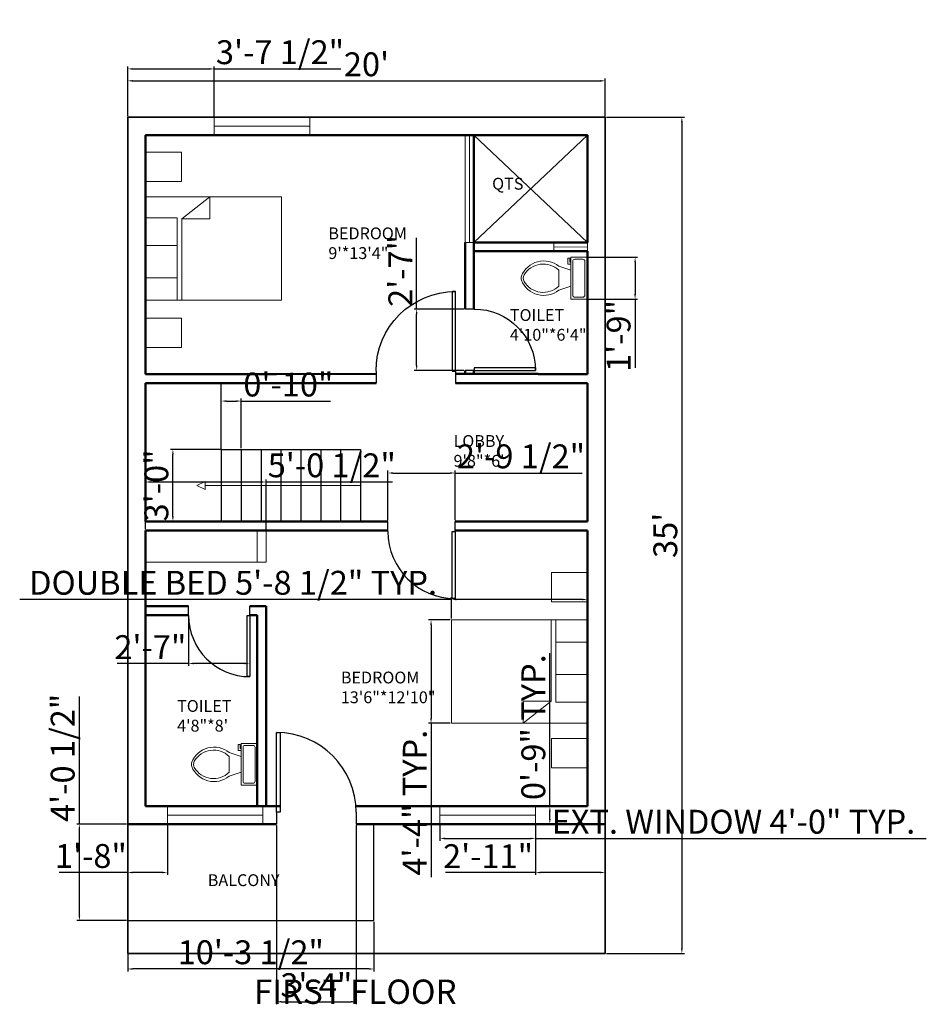
# Model space of a CAD drawing. Units: inches. Extents: x 2157 to 3060, y 2058 to 2553.
# Tile 2 of 2: x 2604 to 3060, y 2058 to 2553. Entities that reach past the tile are written whole.
import ezdxf

# ---------------------------------------------------------------- set-up
doc = ezdxf.new("R2010")
doc.units = ezdxf.units.IN
for name, color, linetype, lineweight in [('A-ANNO-DIMS', 2, 'Continuous', 18), ('A-ANNO-SYMB', 7, 'Continuous', 13), ('A-ANNO-TEXT', 7, 'Continuous', 35), ('A-AREA-IDEN', 7, 'Continuous', 18), ('A-FLOR', 7, 'Continuous', 25), ('A-FLOR-CASE', 32, 'Continuous', 20), ('A-FLOR-FIXT', 9, 'Continuous', 18), ('A-FLOR-STRS', 7, 'Continuous', 25), ('C-PROP', 7, 'Continuous', 35), ('DOOR', 2, 'Continuous', 25), ('FURNITURE', 32, 'Continuous', 18), ('WALL', 7, 'Continuous', 50), ('WINDOW', 130, 'Continuous', 18)]:
    doc.layers.add(name, color=color, linetype=linetype, lineweight=lineweight)
doc.styles.get("Standard").update_dxf_attribs({"font": 'arial.ttf'})
doc.dimstyles.new('ISO-25', dxfattribs={"dimtxt": 12, "dimasz": 2.5, "dimexe": 1.25, "dimexo": 0.625, "dimtad": 1, "dimdec": 0, "dimlunit": 4, "dimtxsty": 'Standard', "dimcen": 2.5, "dimadec": 0, "dimazin": 0, "dimtfac": 1, "dimtdec": 0, "dimtmove": 0, "dimatfit": 3, "dimfxl": 1, "dimarcsym": 0})

# ---------------------------------------------------------------- blocks, each defined once
blk = doc.blocks.new('*U2')
for p, q in [((0, 0), (0, -6)), ((40, 0), (40, -6))]:
    blk.add_line(p, q)
blk.add_lwpolyline([(0, 0), (0, 40), (1.75, 40), (1.75, 0)], close=True)
blk.add_arc((0, 0), 40, 0, 90)
blk = doc.blocks.new('*D7')
at = {"layer": 'A-ANNO-DIMS', "color": 0, "lineweight": -2, "transparency": 16777216}
for p, q in [((2658.57, 2504.59), (2658.57, 2523.53)), ((2898.57, 2504.59), (2898.57, 2523.53)), ((2661.07, 2522.28), (2896.07, 2522.28))]:
    blk.add_line(p, q, dxfattribs=at)
at = {"layer": 'A-ANNO-DIMS', "color": 0, "transparency": 16777216}
for points in [[(2661.07, 2522.7), (2661.07, 2521.86), (2658.57, 2522.28)], [(2896.07, 2522.7), (2896.07, 2521.86), (2898.57, 2522.28)]]:
    blk.add_solid(points, dxfattribs=at)
at = {"layer": 'Defpoints', "color": 0, "transparency": 16777216}
for p in [(2898.57, 2522.28), (2658.57, 2503.96), (2898.57, 2503.96)]:
    blk.add_point(p, dxfattribs=at)
at = {"layer": 'A-ANNO-DIMS', "color": 0, "transparency": 16777216, "insert": (2778.57, 2529.03), "char_height": 12, "attachment_point": 5}
blk.add_mtext("20'", dxfattribs=at)
blk = doc.blocks.new('*D8')
at = {"layer": 'A-ANNO-DIMS', "color": 0, "lineweight": -2, "transparency": 16777216}
for p, q in [((2899.2, 2503.96), (2938.3, 2503.96)), ((2937.05, 2501.46), (2937.05, 2086.46)), ((2899.2, 2083.96), (2938.3, 2083.96))]:
    blk.add_line(p, q, dxfattribs=at)
at = {"layer": 'A-ANNO-DIMS', "color": 0, "transparency": 16777216}
for points in [[(2936.63, 2501.46), (2937.47, 2501.46), (2937.05, 2503.96)], [(2936.63, 2086.46), (2937.47, 2086.46), (2937.05, 2083.96)]]:
    blk.add_solid(points, dxfattribs=at)
at = {"layer": 'Defpoints', "color": 0, "transparency": 16777216}
for p in [(2898.57, 2503.96), (2898.57, 2083.96), (2937.05, 2083.96)]:
    blk.add_point(p, dxfattribs=at)
at = {"layer": 'A-ANNO-DIMS', "color": 0, "transparency": 16777216, "insert": (2930.29, 2293.96), "char_height": 12, "attachment_point": 5, "rotation": 90}
blk.add_mtext("35'", dxfattribs=at)
blk = doc.blocks.new('*U4')
for p, q in [((9.5, -6), (9.5, -2)), ((-10, -8.5), (-8, -8.5)), ((-10, -9.5), (-10, -8.5)), ((-7, -9.5), (-10, -9.5)), ((-8, -8.5), (-8, -8)), ((-7, -8), (-7, -9.5)), ((-4, -8), (-6, -14)), ((4, -8), (6, -14)), ((4, -14), (-4, -14))]:
    blk.add_line(p, q)
blk.add_lwpolyline([(10.5, -8), (10.5, 0), (-10.5, 0), (-10.5, -8)], close=True)
for points in [[(-9.5, -2), (-9.5, -6)], [(8.5, -1), (-8.5, -1)], [(-8.5, -7), (8.5, -7)]]:
    blk.add_lwpolyline(points)
for centre, radius, start, end in [((-8.62, -1.88), 0.884, 81.8699, 188.1301), ((8.62, -1.88), 0.884, 351.8699, 98.1301), ((-8.62, -6.12), 0.884, 171.8699, 278.1301), ((8.62, -6.12), 0.884, 261.8699, 8.1301), ((3.52, -21.58), 12.17, 141.4691, 247.9714), ((4.2, -21.82), 11.33, 136.3677, 238.9468), ((-3.52, -21.58), 12.17, 292.0284, 38.5307), ((-4.2, -21.82), 11.33, 301.053, 43.6321), ((0, -27.88), 4, 245.7318, 294.2682), ((0, -29), 4, 254.8605, 285.1395)]:
    blk.add_arc(centre, radius, start, end)
blk = doc.blocks.new('BED-DOUBLE')
for p, q in [((18.2, 40.88), (32.33, 51.9)), ((32.33, 40.88), (32.33, 51.9)), ((18.2, 0), (18.2, 40.88)), ((18.2, 40.88), (32.33, 40.88)), ((0, 27.39), (15.88, 27.39)), ((0, 11.16), (15.88, 11.16))]:
    blk.add_line(p, q)
for points in [[(0, 0), (68.32, 0), (68.32, 51.9), (0, 51.9)], [(0, 0), (15.88, 0), (15.88, 41.3), (0, 41.3)]]:
    blk.add_lwpolyline(points, close=True)
blk = doc.blocks.new('NIGHTSTAND')
blk.add_lwpolyline([(0, 0), (17.99, 0), (17.99, 14.76), (0, 14.76)], close=True)
blk = doc.blocks.new('STAIR-FLIGHT')
for p, q in [((0, 36.14), (0, 69.5)), ((0, 36.14), (70, 36.14)), ((0, 36.14), (0, 0)), ((0, 36.14), (0, 0)), ((0, 36.14), (0, 0)), ((0, 36.14), (0, 0)), ((10, 36.14), (10, 0)), ((10, 36.14), (10, 0)), ((10, 36.14), (10, 0)), ((10, 36.14), (10, 0)), ((20, 36.14), (20, 0)), ((30, 36.14), (30, 0)), ((30, 36.14), (30, 0)), ((30, 36.14), (30, 0)), ((30, 36.14), (30, 0)), ((40, 36.14), (40, 0)), ((50, 36.14), (50, 0)), ((50, 36.14), (50, 0)), ((50, 36.14), (50, 0)), ((50, 36.14), (50, 0)), ((60, 36.14), (60, 0)), ((70, 36.14), (70, 0))]:
    blk.add_line(p, q)
blk = doc.blocks.new('STAIR-DIRECTION')
for p, q in [((4.17, 4), (0, 2)), ((0, 2), (4.17, 0)), ((4.17, 0), (4.17, 4)), ((82.21, 2), (4.17, 2)), ((4.17, 2), (4.17, 0))]:
    blk.add_line(p, q)
blk = doc.blocks.new('WIN-48IN-EXT')
for p, q in [((0, 4.5), (0, 9)), ((48, 4.5), (48, 9)), ((0, 4.5), (0, 0)), ((0, 4.5), (48, 4.5)), ((48, 4.5), (48, 0))]:
    blk.add_line(p, q)
blk = doc.blocks.new('OPEN-TO-SKY-MARK')
for p, q in [((57, 53.82), (0, 0)), ((57, 0), (0, 53.82))]:
    blk.add_line(p, q)
blk = doc.blocks.new('*D17')
at = {"layer": 'A-ANNO-DIMS', "color": 0, "lineweight": -2, "transparency": 16777216}
for p, q in [((2821.26, 2261.73), (2604.28, 2261.73)), ((2821.26, 2252.11), (2821.26, 2262.98)), ((2887.07, 2261.73), (2823.76, 2261.73)), ((2889.57, 2252.11), (2889.57, 2262.98))]:
    blk.add_line(p, q, dxfattribs=at)
at = {"layer": 'A-ANNO-DIMS', "color": 0, "transparency": 16777216}
for points in [[(2823.76, 2262.15), (2823.76, 2261.31), (2821.26, 2261.73)], [(2887.07, 2262.15), (2887.07, 2261.31), (2889.57, 2261.73)]]:
    blk.add_solid(points, dxfattribs=at)
at = {"layer": 'Defpoints', "color": 0, "transparency": 16777216}
for p in [(2821.26, 2261.73), (2821.26, 2251.48), (2889.57, 2251.48)]:
    blk.add_point(p, dxfattribs=at)
at = {"layer": 'A-ANNO-DIMS', "color": 0, "transparency": 16777216, "insert": (2711.52, 2268.57), "char_height": 12, "attachment_point": 5}
blk.add_mtext('DOUBLE BED 5\'-8 1/2" TYP.', dxfattribs=at)
blk = doc.blocks.new('*D18')
at = {"layer": 'A-ANNO-DIMS', "color": 0, "lineweight": -2, "transparency": 16777216}
for p, q in [((2820.63, 2251.48), (2809.76, 2251.48)), ((2811.01, 2248.98), (2811.01, 2202.09)), ((2820.63, 2199.59), (2809.76, 2199.59)), ((2811.01, 2199.59), (2811.01, 2122.21))]:
    blk.add_line(p, q, dxfattribs=at)
at = {"layer": 'A-ANNO-DIMS', "color": 0, "transparency": 16777216}
for points in [[(2810.59, 2248.98), (2811.43, 2248.98), (2811.01, 2251.48)], [(2810.59, 2202.09), (2811.43, 2202.09), (2811.01, 2199.59)]]:
    blk.add_solid(points, dxfattribs=at)
at = {"layer": 'Defpoints', "color": 0, "transparency": 16777216}
for p in [(2821.26, 2251.48), (2811.01, 2199.59), (2821.26, 2199.59)]:
    blk.add_point(p, dxfattribs=at)
at = {"layer": 'A-ANNO-DIMS', "color": 0, "transparency": 16777216, "insert": (2804.38, 2159.65), "char_height": 12, "attachment_point": 5, "rotation": 90}
blk.add_mtext('4\'-4" TYP.', dxfattribs=at)
blk = doc.blocks.new('*D19')
at = {"layer": 'A-ANNO-DIMS', "color": 0, "lineweight": -2, "transparency": 16777216}
for p, q in [((2815.5, 2148.26), (2815.5, 2140.43)), ((2863.5, 2148.26), (2863.5, 2140.43)), ((2818, 2141.68), (2861, 2141.68)), ((2863.5, 2141.68), (3059.9, 2141.68))]:
    blk.add_line(p, q, dxfattribs=at)
at = {"layer": 'A-ANNO-DIMS', "color": 0, "transparency": 16777216}
for points in [[(2818, 2142.1), (2818, 2141.26), (2815.5, 2141.68)], [(2861, 2142.1), (2861, 2141.26), (2863.5, 2141.68)]]:
    blk.add_solid(points, dxfattribs=at)
at = {"layer": 'Defpoints', "color": 0, "transparency": 16777216}
for p in [(2815.5, 2148.88), (2863.5, 2148.88), (2863.5, 2141.68)]:
    blk.add_point(p, dxfattribs=at)
at = {"layer": 'A-ANNO-DIMS', "color": 0, "transparency": 16777216, "insert": (2962.95, 2148.52), "char_height": 12, "attachment_point": 5}
blk.add_mtext('EXT. WINDOW 4\'-0" TYP.', dxfattribs=at)
blk = doc.blocks.new('*D20')
at = {"layer": 'A-ANNO-DIMS', "color": 0, "lineweight": -2, "transparency": 16777216}
for p, q in [((2870.7, 2157.88), (2870.7, 2234.78)), ((2864.13, 2157.88), (2871.95, 2157.88)), ((2870.7, 2151.38), (2870.7, 2155.38)), ((2864.13, 2148.88), (2871.95, 2148.88))]:
    blk.add_line(p, q, dxfattribs=at)
at = {"layer": 'A-ANNO-DIMS', "color": 0, "transparency": 16777216}
for points in [[(2870.29, 2155.38), (2871.12, 2155.38), (2870.7, 2157.88)], [(2870.29, 2151.38), (2871.12, 2151.38), (2870.7, 2148.88)]]:
    blk.add_solid(points, dxfattribs=at)
at = {"layer": 'Defpoints', "color": 0, "transparency": 16777216}
for p in [(2863.5, 2157.88), (2870.7, 2157.88), (2863.5, 2148.88)]:
    blk.add_point(p, dxfattribs=at)
at = {"layer": 'A-ANNO-DIMS', "color": 0, "transparency": 16777216, "insert": (2863.95, 2197.58), "char_height": 12, "attachment_point": 5, "rotation": 90}
blk.add_mtext('0\'-9" TYP.', dxfattribs=at)
blk = doc.blocks.new('*D25')
at = {"layer": 'A-ANNO-DIMS', "color": 0, "lineweight": -2, "transparency": 16777216}
for p, q in [((2658.57, 2099.79), (2658.57, 2074.86)), ((2782.27, 2099.79), (2782.27, 2074.86)), ((2779.77, 2076.11), (2661.07, 2076.11))]:
    blk.add_line(p, q, dxfattribs=at)
at = {"layer": 'A-ANNO-DIMS', "color": 0, "transparency": 16777216}
for points in [[(2661.07, 2076.53), (2661.07, 2075.7), (2658.57, 2076.11)], [(2779.77, 2076.53), (2779.77, 2075.7), (2782.27, 2076.11)]]:
    blk.add_solid(points, dxfattribs=at)
at = {"layer": 'Defpoints', "color": 0, "transparency": 16777216}
for p in [(2658.57, 2100.41), (2782.27, 2100.41), (2658.57, 2076.11)]:
    blk.add_point(p, dxfattribs=at)
at = {"layer": 'A-ANNO-DIMS', "color": 0, "transparency": 16777216, "insert": (2720.42, 2082.95), "char_height": 12, "attachment_point": 5}
blk.add_mtext('10\'-3 1/2"', dxfattribs=at)
blk = doc.blocks.new('*D26')
at = {"layer": 'A-ANNO-DIMS', "color": 0, "lineweight": -2, "transparency": 16777216}
for p, q in [((2634.27, 2148.88), (2634.27, 2212.98)), ((2657.95, 2148.88), (2633.02, 2148.88)), ((2634.27, 2102.91), (2634.27, 2146.38)), ((2657.95, 2100.41), (2633.02, 2100.41))]:
    blk.add_line(p, q, dxfattribs=at)
at = {"layer": 'A-ANNO-DIMS', "color": 0, "transparency": 16777216}
for points in [[(2633.86, 2146.38), (2634.69, 2146.38), (2634.27, 2148.88)], [(2633.86, 2102.91), (2634.69, 2102.91), (2634.27, 2100.41)]]:
    blk.add_solid(points, dxfattribs=at)
at = {"layer": 'Defpoints', "color": 0, "transparency": 16777216}
for p in [(2634.27, 2148.88), (2658.57, 2148.88), (2658.57, 2100.41)]:
    blk.add_point(p, dxfattribs=at)
at = {"layer": 'A-ANNO-DIMS', "color": 0, "transparency": 16777216, "insert": (2627.44, 2182.18), "char_height": 12, "attachment_point": 5, "rotation": 90}
blk.add_mtext('4\'-0 1/2"', dxfattribs=at)
blk = doc.blocks.new('*D28')
at = {"layer": 'A-ANNO-DIMS', "color": 0, "lineweight": -2, "transparency": 16777216}
for p, q in [((2733.35, 2148.26), (2733.35, 2058.41)), ((2773.35, 2148.26), (2773.35, 2058.41)), ((2735.85, 2059.66), (2770.85, 2059.66))]:
    blk.add_line(p, q, dxfattribs=at)
at = {"layer": 'A-ANNO-DIMS', "color": 0, "transparency": 16777216}
for points in [[(2735.85, 2060.08), (2735.85, 2059.25), (2733.35, 2059.66)], [(2770.85, 2060.08), (2770.85, 2059.25), (2773.35, 2059.66)]]:
    blk.add_solid(points, dxfattribs=at)
at = {"layer": 'Defpoints', "color": 0, "transparency": 16777216}
for p in [(2733.35, 2148.88), (2773.35, 2148.88), (2773.35, 2059.66)]:
    blk.add_point(p, dxfattribs=at)
at = {"layer": 'A-ANNO-DIMS', "color": 0, "transparency": 16777216, "insert": (2753.35, 2066.42), "char_height": 12, "attachment_point": 5}
blk.add_mtext('3\'-4"', dxfattribs=at)
blk = doc.blocks.new('*D31')
at = {"layer": 'A-ANNO-DIMS', "color": 0, "lineweight": -2, "transparency": 16777216}
for p, q in [((2658.57, 2504.59), (2658.57, 2529.51)), ((2661.07, 2528.26), (2699.56, 2528.26)), ((2702.06, 2504.59), (2702.06, 2529.51)), ((2702.06, 2528.26), (2765.66, 2528.26))]:
    blk.add_line(p, q, dxfattribs=at)
at = {"layer": 'A-ANNO-DIMS', "color": 0, "transparency": 16777216}
for points in [[(2661.07, 2528.68), (2661.07, 2527.85), (2658.57, 2528.26)], [(2699.56, 2528.68), (2699.56, 2527.85), (2702.06, 2528.26)]]:
    blk.add_solid(points, dxfattribs=at)
at = {"layer": 'Defpoints', "color": 0, "transparency": 16777216}
for p in [(2702.06, 2528.26), (2658.57, 2503.96), (2702.06, 2503.96)]:
    blk.add_point(p, dxfattribs=at)
at = {"layer": 'A-ANNO-DIMS', "color": 0, "transparency": 16777216, "insert": (2735.11, 2535.1), "char_height": 12, "attachment_point": 5}
blk.add_mtext('3\'-7 1/2"', dxfattribs=at)
blk = doc.blocks.new('*D34')
at = {"layer": 'A-ANNO-DIMS', "color": 0, "lineweight": -2, "transparency": 16777216}
for p, q in [((2658.57, 2148.26), (2658.57, 2123.33)), ((2678.52, 2148.26), (2678.52, 2123.33)), ((2658.57, 2124.58), (2624.05, 2124.58)), ((2676.02, 2124.58), (2661.07, 2124.58))]:
    blk.add_line(p, q, dxfattribs=at)
at = {"layer": 'A-ANNO-DIMS', "color": 0, "transparency": 16777216}
for points in [[(2661.07, 2125), (2661.07, 2124.16), (2658.57, 2124.58)], [(2676.02, 2125), (2676.02, 2124.16), (2678.52, 2124.58)]]:
    blk.add_solid(points, dxfattribs=at)
at = {"layer": 'Defpoints', "color": 0, "transparency": 16777216}
for p in [(2658.57, 2148.88), (2678.52, 2148.88), (2658.57, 2124.58)]:
    blk.add_point(p, dxfattribs=at)
at = {"layer": 'A-ANNO-DIMS', "color": 0, "transparency": 16777216, "insert": (2640.06, 2131.33), "char_height": 12, "attachment_point": 5}
blk.add_mtext('1\'-8"', dxfattribs=at)
blk = doc.blocks.new('*D35')
at = {"layer": 'A-ANNO-DIMS', "color": 0, "lineweight": -2, "transparency": 16777216}
for p, q in [((2863.5, 2148.26), (2863.5, 2123.33)), ((2898.57, 2148.26), (2898.57, 2123.33)), ((2863.5, 2124.58), (2818.33, 2124.58)), ((2896.07, 2124.58), (2866, 2124.58))]:
    blk.add_line(p, q, dxfattribs=at)
at = {"layer": 'A-ANNO-DIMS', "color": 0, "transparency": 16777216}
for points in [[(2866, 2125), (2866, 2124.16), (2863.5, 2124.58)], [(2896.07, 2125), (2896.07, 2124.16), (2898.57, 2124.58)]]:
    blk.add_solid(points, dxfattribs=at)
at = {"layer": 'Defpoints', "color": 0, "transparency": 16777216}
for p in [(2863.5, 2148.88), (2898.57, 2148.88), (2863.5, 2124.58)]:
    blk.add_point(p, dxfattribs=at)
at = {"layer": 'A-ANNO-DIMS', "color": 0, "transparency": 16777216, "insert": (2839.67, 2131.23), "char_height": 12, "attachment_point": 5}
blk.add_mtext('2\'-11"', dxfattribs=at)
blk = doc.blocks.new('*D39')
at = {"layer": 'A-ANNO-DIMS', "color": 0, "lineweight": -2, "transparency": 16777216}
for p, q in [((2789.36, 2301.59), (2789.36, 2326.51)), ((2791.86, 2325.26), (2820.56, 2325.26)), ((2823.06, 2301.59), (2823.06, 2326.51)), ((2823.06, 2325.26), (2886.88, 2325.26))]:
    blk.add_line(p, q, dxfattribs=at)
at = {"layer": 'A-ANNO-DIMS', "color": 0, "transparency": 16777216}
for points in [[(2791.86, 2325.68), (2791.86, 2324.85), (2789.36, 2325.26)], [(2820.56, 2325.68), (2820.56, 2324.85), (2823.06, 2325.26)]]:
    blk.add_solid(points, dxfattribs=at)
at = {"layer": 'Defpoints', "color": 0, "transparency": 16777216}
for p in [(2823.06, 2325.26), (2789.36, 2300.96), (2823.06, 2300.96)]:
    blk.add_point(p, dxfattribs=at)
at = {"layer": 'A-ANNO-DIMS', "color": 0, "transparency": 16777216, "insert": (2856.22, 2332.09), "char_height": 12, "attachment_point": 5}
blk.add_mtext('2\'-9 1/2"', dxfattribs=at)
blk = doc.blocks.new('*D40')
at = {"layer": 'A-ANNO-DIMS', "color": 0, "lineweight": -2, "transparency": 16777216}
for p, q in [((2803.77, 2407.62), (2803.77, 2443.47)), ((2827.45, 2407.62), (2802.52, 2407.62)), ((2803.77, 2379.32), (2803.77, 2405.12)), ((2827.45, 2376.82), (2802.52, 2376.82))]:
    blk.add_line(p, q, dxfattribs=at)
at = {"layer": 'A-ANNO-DIMS', "color": 0, "transparency": 16777216}
for points in [[(2803.36, 2405.12), (2804.19, 2405.12), (2803.77, 2407.62)], [(2803.36, 2379.32), (2804.19, 2379.32), (2803.77, 2376.82)]]:
    blk.add_solid(points, dxfattribs=at)
at = {"layer": 'Defpoints', "color": 0, "transparency": 16777216}
for p in [(2803.77, 2407.62), (2828.07, 2407.62), (2828.07, 2376.82)]:
    blk.add_point(p, dxfattribs=at)
at = {"layer": 'A-ANNO-DIMS', "color": 0, "transparency": 16777216, "insert": (2797.12, 2426.8), "char_height": 12, "attachment_point": 5, "rotation": 90}
blk.add_mtext('2\'-7"', dxfattribs=at)
blk = doc.blocks.new('*D45')
at = {"layer": 'A-ANNO-DIMS', "color": 0, "lineweight": -2, "transparency": 16777216}
for p, q in [((2705.57, 2337.73), (2705.57, 2362.66)), ((2708.07, 2361.41), (2713.07, 2361.41)), ((2715.57, 2337.73), (2715.57, 2362.66)), ((2715.57, 2361.41), (2760.55, 2361.41))]:
    blk.add_line(p, q, dxfattribs=at)
at = {"layer": 'A-ANNO-DIMS', "color": 0, "transparency": 16777216}
for points in [[(2708.07, 2361.82), (2708.07, 2360.99), (2705.57, 2361.41)], [(2713.07, 2361.82), (2713.07, 2360.99), (2715.57, 2361.41)]]:
    blk.add_solid(points, dxfattribs=at)
at = {"layer": 'Defpoints', "color": 0, "transparency": 16777216}
for p in [(2715.57, 2361.41), (2705.57, 2337.11), (2715.57, 2337.11)]:
    blk.add_point(p, dxfattribs=at)
at = {"layer": 'A-ANNO-DIMS', "color": 0, "transparency": 16777216, "insert": (2739.31, 2368.16), "char_height": 12, "attachment_point": 5}
blk.add_mtext('0\'-10"', dxfattribs=at)
blk = doc.blocks.new('*D46')
at = {"layer": 'A-ANNO-DIMS', "color": 0, "lineweight": -2, "transparency": 16777216}
for p, q in [((2704.95, 2337.11), (2680.02, 2337.11)), ((2681.27, 2303.46), (2681.27, 2334.61)), ((2704.95, 2300.96), (2680.02, 2300.96))]:
    blk.add_line(p, q, dxfattribs=at)
at = {"layer": 'A-ANNO-DIMS', "color": 0, "transparency": 16777216}
for points in [[(2680.86, 2334.61), (2681.69, 2334.61), (2681.27, 2337.11)], [(2680.86, 2303.46), (2681.69, 2303.46), (2681.27, 2300.96)]]:
    blk.add_solid(points, dxfattribs=at)
at = {"layer": 'Defpoints', "color": 0, "transparency": 16777216}
for p in [(2681.27, 2337.11), (2705.57, 2337.11), (2705.57, 2300.96)]:
    blk.add_point(p, dxfattribs=at)
at = {"layer": 'A-ANNO-DIMS', "color": 0, "transparency": 16777216, "insert": (2674.52, 2319.03), "char_height": 12, "attachment_point": 5, "rotation": 90}
blk.add_mtext('3\'-0"', dxfattribs=at)
blk = doc.blocks.new('*D49')
at = {"layer": 'A-ANNO-DIMS', "color": 0, "lineweight": -2, "transparency": 16777216}
for p, q in [((2689.13, 2253.26), (2689.13, 2228.33)), ((2719.92, 2253.26), (2719.92, 2228.33)), ((2689.13, 2229.58), (2653.28, 2229.58)), ((2717.42, 2229.58), (2691.63, 2229.58))]:
    blk.add_line(p, q, dxfattribs=at)
at = {"layer": 'A-ANNO-DIMS', "color": 0, "transparency": 16777216}
for points in [[(2691.63, 2230), (2691.63, 2229.16), (2689.13, 2229.58)], [(2717.42, 2230), (2717.42, 2229.16), (2719.92, 2229.58)]]:
    blk.add_solid(points, dxfattribs=at)
at = {"layer": 'Defpoints', "color": 0, "transparency": 16777216}
for p in [(2689.13, 2253.88), (2719.92, 2253.88), (2689.13, 2229.58)]:
    blk.add_point(p, dxfattribs=at)
at = {"layer": 'A-ANNO-DIMS', "color": 0, "transparency": 16777216, "insert": (2669.95, 2236.23), "char_height": 12, "attachment_point": 5}
blk.add_mtext('2\'-7"', dxfattribs=at)
blk = doc.blocks.new('*D50')
at = {"layer": 'A-ANNO-DIMS', "color": 0, "lineweight": -2, "transparency": 16777216}
for p, q in [((2889.87, 2433.63), (2914.8, 2433.63)), ((2913.55, 2431.13), (2913.55, 2415.13)), ((2889.87, 2412.63), (2914.8, 2412.63)), ((2913.55, 2412.63), (2913.55, 2378.11))]:
    blk.add_line(p, q, dxfattribs=at)
at = {"layer": 'A-ANNO-DIMS', "color": 0, "transparency": 16777216}
for points in [[(2913.13, 2431.13), (2913.97, 2431.13), (2913.55, 2433.63)], [(2913.13, 2415.13), (2913.97, 2415.13), (2913.55, 2412.63)]]:
    blk.add_solid(points, dxfattribs=at)
at = {"layer": 'Defpoints', "color": 0, "transparency": 16777216}
for p in [(2889.25, 2433.63), (2889.25, 2412.63), (2913.55, 2412.63)]:
    blk.add_point(p, dxfattribs=at)
at = {"layer": 'A-ANNO-DIMS', "color": 0, "transparency": 16777216, "insert": (2906.8, 2394.12), "char_height": 12, "attachment_point": 5, "rotation": 90}
blk.add_mtext('1\'-9"', dxfattribs=at)
blk = doc.blocks.new('*D51')
at = {"layer": 'A-ANNO-DIMS', "color": 0, "lineweight": -2, "transparency": 16777216}
for p, q in [((2667.57, 2297.09), (2667.57, 2322.01)), ((2670.07, 2320.76), (2725.57, 2320.76)), ((2728.07, 2297.09), (2728.07, 2322.01)), ((2728.07, 2320.76), (2791.68, 2320.76))]:
    blk.add_line(p, q, dxfattribs=at)
at = {"layer": 'A-ANNO-DIMS', "color": 0, "transparency": 16777216}
for points in [[(2670.07, 2321.18), (2670.07, 2320.35), (2667.57, 2320.76)], [(2725.57, 2321.18), (2725.57, 2320.35), (2728.07, 2320.76)]]:
    blk.add_solid(points, dxfattribs=at)
at = {"layer": 'Defpoints', "color": 0, "transparency": 16777216}
for p in [(2728.07, 2320.76), (2667.57, 2296.46), (2728.07, 2296.46)]:
    blk.add_point(p, dxfattribs=at)
at = {"layer": 'A-ANNO-DIMS', "color": 0, "transparency": 16777216, "insert": (2761.13, 2327.59), "char_height": 12, "attachment_point": 5}
blk.add_mtext('5\'-0 1/2"', dxfattribs=at)

msp = doc.modelspace()

# ---------------------------------------------------------------- linework, layer by layer
at = {"layer": 'A-FLOR'}
for p, q in [((2782.27, 2100.41), (2782.27, 2148.88)), ((2658.57, 2100.41), (2782.27, 2100.41))]:
    msp.add_line(p, q, dxfattribs=at)
at = {"layer": 'A-FLOR-CASE'}
for p, q in [((2723.57, 2280.44), (2723.57, 2296.46)), ((2728.07, 2296.46), (2728.07, 2280.44)), ((2728.07, 2280.44), (2667.57, 2280.44)), ((2667.57, 2280.44), (2723.57, 2280.44))]:
    msp.add_line(p, q, dxfattribs=at)
at = {"layer": 'C-PROP'}
msp.add_lwpolyline([(2658.57, 2083.96), (2898.57, 2083.96), (2898.57, 2503.96), (2658.57, 2503.96)], close=True, dxfattribs=at)
at = {"layer": 'WALL'}
for p, q in [((2667.57, 2494.96), (2775.57, 2494.96)), ((2775.57, 2494.96), (2823.57, 2494.96)), ((2832.57, 2494.96), (2832.57, 2407.62)), ((2889.57, 2441.14), (2889.57, 2494.96)), ((2828.07, 2441.14), (2828.07, 2407.62)), ((2832.57, 2441.14), (2889.57, 2441.14)), ((2832.57, 2436.64), (2889.57, 2436.64)), ((2889.57, 2374.96), (2889.57, 2436.64)), ((2733.32, 2374.96), (2667.57, 2374.96)), ((2733.32, 2374.96), (2783.35, 2375.01)), ((2823.35, 2375.04), (2864.82, 2375.08)), ((2828.07, 2376.82), (2828.07, 2374.96)), ((2832.57, 2376.82), (2832.57, 2375.05)), ((2864.82, 2374.96), (2889.57, 2374.96)), ((2733.32, 2370.46), (2667.57, 2370.46)), ((2783.35, 2370.46), (2733.32, 2370.46)), ((2864.82, 2370.46), (2823.35, 2370.46)), ((2832.57, 2370.46), (2834.02, 2370.46)), ((2864.82, 2370.46), (2889.57, 2370.46)), ((2667.57, 2300.96), (2775.57, 2300.96)), ((2775.57, 2300.96), (2789.36, 2300.96)), ((2823.06, 2300.96), (2889.57, 2300.96)), ((2667.57, 2192.96), (2667.57, 2296.46)), ((2667.57, 2296.46), (2771.07, 2296.46)), ((2789.36, 2296.46), (2767.15, 2296.46)), ((2889.57, 2296.46), (2823.06, 2296.46)), ((2689.13, 2258.38), (2667.57, 2258.38)), ((2728.07, 2258.38), (2719.92, 2258.38)), ((2728.07, 2157.88), (2728.07, 2258.38)), ((2689.13, 2253.88), (2667.57, 2253.88)), ((2723.57, 2253.88), (2719.92, 2253.88)), ((2723.57, 2157.88), (2723.57, 2253.88)), ((2667.57, 2197.46), (2667.57, 2221.46)), ((2667.57, 2192.96), (2667.57, 2157.88)), ((2735.1, 2157.88), (2667.57, 2157.88)), ((2667.57, 2157.88), (2723.57, 2157.88)), ((2779.57, 2157.88), (2773.24, 2157.88)), ((2779.57, 2157.88), (2889.57, 2157.88)), ((2733.35, 2148.88), (2658.57, 2148.88)), ((2773.35, 2148.88), (2779.57, 2148.88)), ((2779.57, 2148.88), (2889.57, 2148.88)), ((2889.57, 2148.88), (2898.57, 2148.88))]:
    msp.add_line(p, q, dxfattribs=at)
for points in [[(2889.57, 2441.14), (2889.57, 2494.96), (2667.57, 2494.96), (2667.57, 2374.96)], [(2889.57, 2374.96), (2889.57, 2436.64)], [(2667.57, 2370.46), (2667.57, 2300.96)], [(2889.57, 2300.96), (2889.57, 2370.46)], [(2667.57, 2296.46), (2667.57, 2192.96)], [(2889.57, 2157.88), (2889.57, 2296.46)]]:
    msp.add_lwpolyline(points, dxfattribs=at)
at = {"layer": 'WINDOW'}
for p, q in [((2828.07, 2450.46), (2828.07, 2494.96)), ((2830.32, 2441.14), (2830.32, 2494.96)), ((2828.07, 2450.46), (2828.07, 2441.14)), ((2832.57, 2441.14), (2828.07, 2441.14)), ((2872.71, 2441.14), (2872.71, 2436.64)), ((2872.71, 2438.85), (2889.57, 2438.71)), ((2889.57, 2441.14), (2889.57, 2436.28))]:
    msp.add_line(p, q, dxfattribs=at)

# ---------------------------------------------------------------- block references
at = {"layer": 'A-ANNO-SYMB', "rotation": 180}
msp.add_blockref('OPEN-TO-SKY-MARK', (2889.57, 2494.96), dxfattribs=at)
at = {"layer": 'A-ANNO-SYMB'}
msp.add_blockref('STAIR-DIRECTION', (2693.36, 2317.04), dxfattribs=at)
at = {"layer": 'A-FLOR-FIXT', "rotation": 270}
for p in [(2889.25, 2423.13), (2723.57, 2178.91)]:
    msp.add_blockref('*U4', p, dxfattribs=at)
at = {"layer": 'A-FLOR-STRS'}
msp.add_blockref('STAIR-FLIGHT', (2705.57, 2300.96), dxfattribs=at)
at = {"layer": 'DOOR', "xscale": -1}
msp.add_blockref('*U2', (2823.35, 2376.46), dxfattribs=at)
at = {"layer": 'DOOR'}
for p, xscale, yscale, zscale, rotation in [((2832.69, 2376.82), -0.7698686144923367, 0.7698686144923367, 0.7698686144923367, 270), ((2823.06, 2295.91), 0.8426282986738574, 0.8426282986738574, 0.8426282986738574, 180), ((2719.92, 2253.76), 0.7698686144923367, 0.7698686144923367, 0.7698686144923367, 180)]:
    msp.add_blockref('*U2', p, dxfattribs=dict(at, xscale=xscale, yscale=yscale, zscale=zscale, rotation=rotation))
msp.add_blockref('*U2', (2733.35, 2154.88), dxfattribs=at)
at = {"layer": 'FURNITURE'}
for name, p in [('NIGHTSTAND', (2667.57, 2471.73)), ('BED-DOUBLE', (2667.57, 2412.1)), ('NIGHTSTAND', (2667.57, 2388.26))]:
    msp.add_blockref(name, p, dxfattribs=at)
at = {"layer": 'FURNITURE', "rotation": 180}
for name, p in [('NIGHTSTAND', (2889.57, 2275.32)), ('BED-DOUBLE', (2889.57, 2251.48)), ('NIGHTSTAND', (2889.57, 2191.85))]:
    msp.add_blockref(name, p, dxfattribs=at)
at = {"layer": 'WINDOW'}
for p in [(2702.06, 2494.96), (2678.52, 2148.88), (2815.5, 2148.88)]:
    msp.add_blockref('WIN-48IN-EXT', p, dxfattribs=at)

# ---------------------------------------------------------------- texts
at = {"layer": 'A-ANNO-TEXT', "insert": (2722.02, 2070.8), "char_height": 12.2084, "attachment_point": 1}
msp.add_mtext_dynamic_manual_height_columns('FIRST FLOOR', width=597.5375, gutter_width=61.04, heights=[0], dxfattribs=at)
at = {"layer": 'A-AREA-IDEN', "attachment_point": 1}
for s, heights, insert, char_height in [('QTS', [0], (2841.71, 2473.56), 5.949), ('BEDROOM\\P9\'*13\'4"', [0], (2759.4, 2448.63), 5.949), ('TOILET\\P4\'10"*6\'4"', [0], (2850.62, 2407.59), 5.949), ('LOBBY\\P9\'8"*6\'', [0], (2822.31, 2344.3), 5.949), ('BEDROOM\\P13\'6"*12\'10"', [0], (2765.69, 2225.5), 5.9493), ('TOILET \\P4\'8"*8\'', [16.1], (2683.38, 2211.22), 5.949), ('BALCONY', [0], (2698.81, 2123.7), 5.949)]:
    msp.add_mtext_dynamic_manual_height_columns(s, width=65.8339, gutter_width=29.75, heights=heights, dxfattribs=dict(at, insert=insert, char_height=char_height))

# ---------------------------------------------------------------- dimensions: what is measured, and where the dimension line sits
at = {"layer": 'A-ANNO-DIMS'}
for base, p1, p2, override, picture, middle in [((2702.06, 2528.26), (2658.57, 2503.96), (2702.06, 2503.96), {"dimdec": 1, "dimlfac": 1, "dimrnd": 0, "dimzin": 1, "dimdsep": 46, "dimlunit": 4, "dimfrac": 2}, '*D31', (2735.11, 2535.1)), ((2898.57, 2522.28), (2658.57, 2503.96), (2898.57, 2503.96), {"dimclrd": 0, "dimclre": 0, "dimclrt": 0}, '*D7', (2778.57, 2529.03)), ((2715.57, 2361.41), (2705.57, 2337.11), (2715.57, 2337.11), {"dimdec": 1, "dimlfac": 1, "dimrnd": 0, "dimzin": 1, "dimdsep": 46, "dimlunit": 4, "dimfrac": 2}, '*D45', (2739.31, 2368.16)), ((2823.06, 2325.26), (2789.36, 2300.96), (2823.06, 2300.96), {"dimdec": 1, "dimlfac": 1, "dimrnd": 0, "dimzin": 1, "dimdsep": 46, "dimlunit": 4, "dimfrac": 2}, '*D39', (2856.22, 2332.09)), ((2728.07, 2320.76), (2667.57, 2296.46), (2728.07, 2296.46), {"dimdec": 1, "dimlfac": 1, "dimrnd": 0, "dimzin": 1, "dimdsep": 46, "dimlunit": 4, "dimfrac": 2}, '*D51', (2761.13, 2327.59)), ((2773.35, 2059.66), (2733.35, 2148.88), (2773.35, 2148.88), {"dimdec": 1, "dimlfac": 1, "dimrnd": 0, "dimzin": 1, "dimdsep": 46, "dimlunit": 4, "dimfrac": 2}, '*D28', (2753.35, 2066.42))]:
    dim = msp.add_linear_dim(base=base, p1=p1, p2=p2, dimstyle='ISO-25', override=override, dxfattribs=at)
    dim.commit()
    dim.dimension.update_dxf_attribs({"geometry": picture, "text_midpoint": middle})
for base, p1, p2, angle, override, picture, middle in [((2937.05, 2083.96), (2898.57, 2503.96), (2898.57, 2083.96), 90, {"dimclrd": 0, "dimclre": 0, "dimclrt": 0}, '*D8', (2930.29, 2293.96)), ((2803.77, 2407.62), (2828.07, 2376.82), (2828.07, 2407.62), 90, {"dimdec": 1, "dimlfac": 1, "dimrnd": 0, "dimzin": 1, "dimdsep": 46, "dimlunit": 4, "dimfrac": 2}, '*D40', (2797.12, 2426.8)), ((2913.55, 2412.63), (2889.25, 2433.63), (2889.25, 2412.63), 270, {"dimdec": 1, "dimlfac": 1, "dimrnd": 0, "dimzin": 1, "dimdsep": 46, "dimlunit": 4, "dimfrac": 2}, '*D50', (2906.8, 2394.12)), ((2681.2741, 2337.105), (2705.5741, 2300.9617), (2705.5741, 2337.105), 90, {"dimdec": 1, "dimlfac": 1, "dimrnd": 0, "dimzin": 1, "dimdsep": 46, "dimlunit": 4, "dimfrac": 2}, '*D46', (2674.5182, 2319.0333)), ((2689.13, 2229.58), (2719.92, 2253.88), (2689.13, 2253.88), 180, {"dimdec": 1, "dimlfac": 1, "dimrnd": 0, "dimzin": 1, "dimdsep": 46, "dimlunit": 4, "dimfrac": 2}, '*D49', (2669.95, 2236.23)), ((2634.27, 2148.88), (2658.57, 2100.41), (2658.57, 2148.88), 90, {"dimdec": 1, "dimlfac": 1, "dimrnd": 0, "dimzin": 1, "dimdsep": 46, "dimlunit": 4, "dimfrac": 2}, '*D26', (2627.44, 2182.18)), ((2658.5741, 2124.5817), (2678.5187, 2148.8817), (2658.5741, 2148.8817), 180, {"dimdec": 1, "dimlfac": 1, "dimrnd": 0, "dimzin": 1, "dimdsep": 46, "dimlunit": 4, "dimfrac": 2}, '*D34', (2640.0644, 2131.3335)), ((2863.5, 2124.58), (2898.57, 2148.88), (2863.5, 2148.88), 180, {"dimdec": 1, "dimlfac": 1, "dimrnd": 0, "dimzin": 1, "dimdsep": 46, "dimlunit": 4, "dimfrac": 2}, '*D35', (2839.67, 2131.23)), ((2658.57, 2076.11), (2782.27, 2100.41), (2658.57, 2100.41), 180, {"dimdec": 1, "dimlfac": 1, "dimrnd": 0, "dimzin": 1, "dimdsep": 46, "dimlunit": 4, "dimfrac": 2}, '*D25', (2720.42, 2082.95))]:
    dim = msp.add_linear_dim(base=base, p1=p1, p2=p2, angle=angle, dimstyle='ISO-25', override=override, dxfattribs=at)
    dim.commit()
    dim.dimension.update_dxf_attribs({"geometry": picture, "text_midpoint": middle})
for base, p1, p2, angle, text, picture, middle in [((2821.26, 2261.73), (2889.57, 2251.48), (2821.26, 2251.48), 180, 'DOUBLE BED <> TYP.', '*D17', (2711.52, 2268.57)), ((2811.01, 2199.59), (2821.26, 2251.48), (2821.26, 2199.59), 270, '<> TYP.', '*D18', (2804.38, 2159.65)), ((2870.7, 2157.88), (2863.5, 2148.88), (2863.5, 2157.88), 90, '<> TYP.', '*D20', (2863.95, 2197.58))]:
    dim = msp.add_linear_dim(base=base, p1=p1, p2=p2, angle=angle, text=text, dimstyle='ISO-25', override={"dimdec": 1, "dimlfac": 1, "dimrnd": 0, "dimzin": 1, "dimdsep": 46, "dimlunit": 4, "dimfrac": 2}, dxfattribs=at)
    dim.commit()
    dim.dimension.update_dxf_attribs({"geometry": picture, "text_midpoint": middle})
dim = msp.add_linear_dim(base=(2863.5, 2141.68), p1=(2815.5, 2148.88), p2=(2863.5, 2148.88), text='EXT. WINDOW <> TYP.', dimstyle='ISO-25', override={"dimdec": 1, "dimlfac": 1, "dimrnd": 0, "dimzin": 1, "dimdsep": 46, "dimlunit": 4, "dimfrac": 2}, dxfattribs=at)
dim.commit()
dim.dimension.update_dxf_attribs({"geometry": '*D19', "text_midpoint": (2962.95, 2148.52)})

doc.saveas('drawing.dxf')
